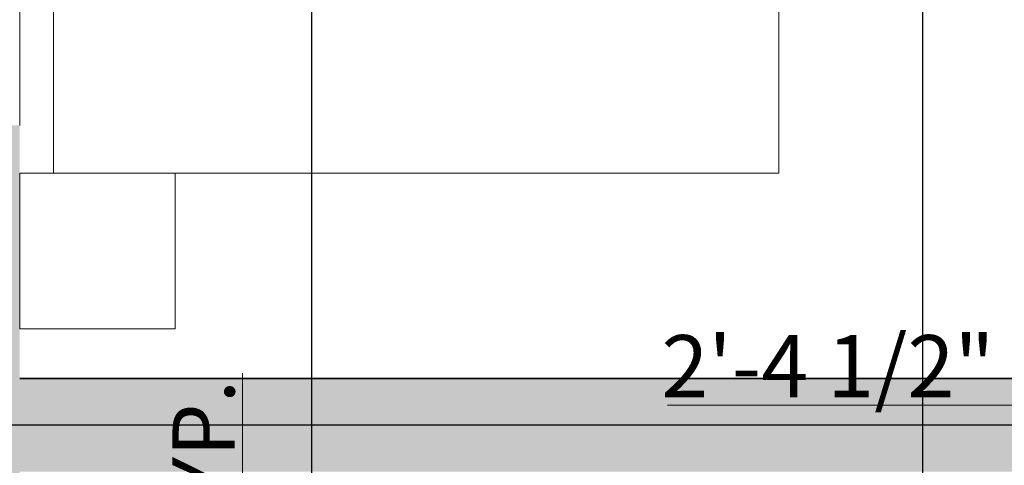
# Model space of a CAD drawing. Units: inches. Extents: x 2696 to 3240, y 1564 to 2310.
# Tile 51 of 76: x 2755 to 2850, y 2137 to 2180. Entities that reach past the tile are written whole.
import ezdxf

# ---------------------------------------------------------------- set-up
doc = ezdxf.new("R2010")
doc.units = ezdxf.units.IN
for name, color, linetype, lineweight in [('A-ANNO-DIMS', 3, 'Continuous', 18), ('A-FURN', 251, 'Continuous', 13), ('A-WALL', 7, 'Continuous', 35), ('A-WALL-PATT', 9, 'Continuous', 13), ('WINDOW', 2, 'Continuous', 18)]:
    doc.layers.add(name, color=color, linetype=linetype, lineweight=lineweight)
doc.styles.add('TIMES NEW', font='times.ttf')
doc.dimstyles.new('Siddhuu', dxfattribs={"dimtxt": 6, "dimasz": 2.5, "dimexe": 1.25, "dimexo": 0.625, "dimtad": 1, "dimdec": 1, "dimlunit": 4, "dimtxsty": 'TIMES NEW', "dimcen": 2.5, "dimclrd": 256, "dimclre": 1, "dimclrt": 7, "dimadec": 0, "dimazin": 0, "dimtfac": 1, "dimtdec": 1, "dimtmove": 0, "dimatfit": 3, "dimfxl": 1, "dimtolj": 1, "dimlwd": -1, "dimarcsym": 0})

# ---------------------------------------------------------------- blocks, each defined once
blk = doc.blocks.new('WD_WIN4')
for p, q in [((-0.5, 0.5), (0.5, 0.5)), ((-0.5, 0.12), (0.5, 0.12)), ((-0.5, -0.12), (0.5, -0.12)), ((-0.5, -0.5), (0.5, -0.5))]:
    blk.add_line(p, q)
blk = doc.blocks.new('BED-DOUBLE-WITH-NIGHTSTANDS')
for points in [[(0, 75.132), (0, 90.158), (15.027, 90.158), (15.027, 75.132)], [(3.281, 15.026), (3.281, 75.132), (73.404, 75.132), (73.404, 15.026)], [(0, 15.026), (0, 0), (15.027, 0), (15.027, 15.026)]]:
    blk.add_lwpolyline(points, close=True)
blk = doc.blocks.new('*D29')
at = {"layer": 'A-ANNO-DIMS', "color": 1, "lineweight": -2, "transparency": 16777216}
for p, q in [((2850.765, 2146.449), (2850.765, 2141.394)), ((2879.111, 2146.449), (2879.111, 2141.394))]:
    blk.add_line(p, q, dxfattribs=at)
at = {"layer": 'A-ANNO-DIMS', "transparency": 16777216}
for p, q in [((2850.765, 2142.644), (2817.236, 2142.644)), ((2876.611, 2142.644), (2853.265, 2142.644))]:
    blk.add_line(p, q, dxfattribs=at)
for points in [[(2853.265, 2143.061), (2853.265, 2142.228), (2850.765, 2142.644)], [(2876.611, 2143.061), (2876.611, 2142.228), (2879.111, 2142.644)]]:
    blk.add_solid(points, dxfattribs=at)
at = {"layer": 'Defpoints', "color": 0, "transparency": 16777216}
for p in [(2850.765, 2147.074), (2879.111, 2147.074), (2850.765, 2142.644)]:
    blk.add_point(p, dxfattribs=at)
at = {"layer": 'A-ANNO-DIMS', "color": 7, "transparency": 16777216, "insert": (2832.75, 2146.406), "char_height": 6, "attachment_point": 5, "style": 'TIMES NEW'}
blk.add_mtext('\\A1;2\'-4 1/2"', dxfattribs=at)
blk = doc.blocks.new('*D41')
at = {"layer": 'A-ANNO-DIMS', "transparency": 16777216}
for p, q in [((2776.142, 2091.201), (2776.142, 2145.728)), ((2776.142, 2087.2), (2776.142, 2088.701))]:
    blk.add_line(p, q, dxfattribs=at)
at = {"layer": 'A-ANNO-DIMS', "color": 1, "lineweight": -2, "transparency": 16777216}
for p, q in [((2776.641, 2091.201), (2774.892, 2091.201)), ((2776.641, 2084.7), (2774.892, 2084.7))]:
    blk.add_line(p, q, dxfattribs=at)
at = {"layer": 'A-ANNO-DIMS', "transparency": 16777216}
for points in [[(2775.725, 2088.701), (2776.558, 2088.701), (2776.142, 2091.201)], [(2775.725, 2087.2), (2776.558, 2087.2), (2776.142, 2084.7)]]:
    blk.add_solid(points, dxfattribs=at)
at = {"layer": 'Defpoints', "color": 0, "transparency": 16777216}
for p in [(2776.142, 2091.201), (2777.266, 2091.201), (2777.266, 2084.7)]:
    blk.add_point(p, dxfattribs=at)
at = {"layer": 'A-ANNO-DIMS', "color": 7, "transparency": 16777216, "insert": (2772.38, 2119.715), "char_height": 6, "attachment_point": 5, "rotation": 90, "style": 'TIMES NEW'}
blk.add_mtext('\\A1;0\'-6 1/2" TYP.', dxfattribs=at)
blk = doc.blocks.new('*D62')
at = {"layer": 'A-ANNO-DIMS', "color": 1, "lineweight": -2, "transparency": 16777216}
for p, q in [((2965.084, 2140.701), (2709.361, 2140.701)), ((2965.084, 2063.591), (2709.361, 2063.591))]:
    blk.add_line(p, q, dxfattribs=at)
at = {"layer": 'A-ANNO-DIMS', "transparency": 16777216}
blk.add_line((2710.611, 2066.091), (2710.611, 2138.201), dxfattribs=at)
for points in [[(2710.195, 2138.201), (2711.028, 2138.201), (2710.611, 2140.701)], [(2710.195, 2066.091), (2711.028, 2066.091), (2710.611, 2063.591)]]:
    blk.add_solid(points, dxfattribs=at)
at = {"layer": 'Defpoints', "color": 0, "transparency": 16777216}
for p in [(2710.611, 2140.701), (2965.709, 2140.701), (2965.709, 2063.591)]:
    blk.add_point(p, dxfattribs=at)
at = {"layer": 'A-ANNO-DIMS', "color": 7, "transparency": 16777216, "insert": (2706.934, 2102.146), "char_height": 6, "attachment_point": 5, "rotation": 90, "style": 'TIMES NEW'}
blk.add_mtext('\\A1;6\'-5"', dxfattribs=at)
blk = doc.blocks.new('*D64')
at = {"layer": 'A-ANNO-DIMS', "color": 1, "lineweight": -2, "transparency": 16777216}
for p, q in [((3073.084, 2206.701), (2709.361, 2206.701)), ((3068.584, 1989.201), (2709.361, 1989.201))]:
    blk.add_line(p, q, dxfattribs=at)
at = {"layer": 'A-ANNO-DIMS', "transparency": 16777216}
blk.add_line((2710.611, 1991.701), (2710.611, 2204.201), dxfattribs=at)
for points in [[(2710.195, 2204.201), (2711.028, 2204.201), (2710.611, 2206.701)], [(2710.195, 1991.701), (2711.028, 1991.701), (2710.611, 1989.201)]]:
    blk.add_solid(points, dxfattribs=at)
at = {"layer": 'Defpoints', "color": 0, "transparency": 16777216}
for p in [(2710.611, 2206.701), (3073.709, 2206.701), (3069.209, 1989.201)]:
    blk.add_point(p, dxfattribs=at)
at = {"layer": 'A-ANNO-DIMS', "color": 7, "transparency": 16777216, "insert": (2706.85, 2097.951), "char_height": 6, "attachment_point": 5, "rotation": 90, "style": 'TIMES NEW'}
blk.add_mtext('\\A1;18\'-1 1/2"', dxfattribs=at)
blk = doc.blocks.new('*D68')
at = {"layer": 'A-ANNO-DIMS', "color": 1, "lineweight": -2, "transparency": 16777216}
for p, q in [((2745.611, 2261.576), (2745.611, 1568.951)), ((2782.834, 2261.576), (2782.834, 1568.951))]:
    blk.add_line(p, q, dxfattribs=at)
at = {"layer": 'A-ANNO-DIMS', "transparency": 16777216}
blk.add_line((2748.111, 1570.201), (2780.334, 1570.201), dxfattribs=at)
for points in [[(2748.111, 1570.618), (2748.111, 1569.784), (2745.611, 1570.201)], [(2780.334, 1570.618), (2780.334, 1569.784), (2782.834, 1570.201)]]:
    blk.add_solid(points, dxfattribs=at)
at = {"layer": 'Defpoints', "color": 0, "transparency": 16777216}
for p in [(2745.611, 2262.201), (2782.834, 2262.201), (2782.834, 1570.201)]:
    blk.add_point(p, dxfattribs=at)
at = {"layer": 'A-ANNO-DIMS', "color": 7, "transparency": 16777216, "insert": (2764.223, 1573.878), "char_height": 6, "attachment_point": 5, "style": 'TIMES NEW'}
blk.add_mtext('\\A1;3\'-1"', dxfattribs=at)
blk = doc.blocks.new('*D69')
at = {"layer": 'A-ANNO-DIMS', "color": 1, "lineweight": -2, "transparency": 16777216}
for p, q in [((2841.889, 2261.576), (2841.889, 1568.951)), ((2905.91, 2261.576), (2905.91, 1568.951))]:
    blk.add_line(p, q, dxfattribs=at)
at = {"layer": 'A-ANNO-DIMS', "transparency": 16777216}
blk.add_line((2844.389, 1570.201), (2903.41, 1570.201), dxfattribs=at)
for points in [[(2844.389, 1570.618), (2844.389, 1569.784), (2841.889, 1570.201)], [(2903.41, 1570.618), (2903.41, 1569.784), (2905.91, 1570.201)]]:
    blk.add_solid(points, dxfattribs=at)
at = {"layer": 'Defpoints', "color": 0, "transparency": 16777216}
for p in [(2841.889, 2262.201), (2905.91, 2262.201), (2905.91, 1570.201)]:
    blk.add_point(p, dxfattribs=at)
at = {"layer": 'A-ANNO-DIMS', "color": 7, "transparency": 16777216, "insert": (2873.9, 1573.878), "char_height": 6, "attachment_point": 5, "style": 'TIMES NEW'}
blk.add_mtext('\\A1;5\'-4"', dxfattribs=at)

msp = doc.modelspace()

# ---------------------------------------------------------------- hatches: boundary and pattern name
at = {"layer": 'A-WALL-PATT', "transparency": 33554556}
h = msp.add_hatch(color=256, dxfattribs=at)
h.dxf.hatch_style = 1
h.paths.add_polyline_path([(2879.111, 2253.201), (2905.91, 2253.201), (2905.91, 2262.201), (2841.889, 2262.201), (2841.889, 2253.201), (2870.111, 2253.201), (2870.111, 2176.601), (2965.709, 2176.601), (2965.709, 2206.701), (2973.583, 2206.701), (2973.583, 2215.701), (2965.709, 2215.701), (2965.709, 2262.201), (2929.91, 2262.201), (2929.91, 2253.201), (2956.709, 2253.201), (2956.709, 2185.601), (2879.111, 2185.601)])
h.paths.add_polyline_path([(2782.834, 2262.201), (2745.611, 2262.201), (2745.611, 2228.729), (2754.611, 2228.729), (2754.611, 2253.201), (2782.834, 2253.201)])
h.paths.add_polyline_path([(2754.611, 2136.201), (2965.709, 2136.201), (2965.709, 2145.201), (2879.111, 2145.201), (2879.111, 2147.074), (2877.34, 2147.074), (2870.111, 2147.074), (2870.111, 2145.201), (2754.611, 2145.201), (2754.611, 2169.674), (2745.611, 2169.674), (2745.611, 2000.201), (2754.611, 2000.201), (2754.611, 2019.201), (2849.083, 2019.201), (2849.083, 2023.701), (2841.209, 2023.701), (2841.209, 2051.827), (2836.709, 2051.827), (2836.709, 2023.701), (2754.611, 2023.701), (2754.611, 2091.201), (2836.709, 2091.201), (2836.709, 2087.827), (2841.209, 2087.827), (2841.209, 2095.701), (2754.611, 2095.701)])
h.paths.add_polyline_path([(2965.709, 2136.201), (2956.709, 2136.201), (2956.709, 2023.701), (2885.083, 2023.701), (2885.083, 2019.201), (2956.709, 2019.201), (2956.709, 1950.575), (2965.709, 1950.575), (2965.709, 1980.201), (2973.583, 1980.201), (2973.583, 1989.201), (2965.709, 1989.201)])
h.paths.add_polyline_path([(2754.611, 1906.701), (2880.209, 1906.701), (2884.709, 1906.701), (2956.709, 1906.701), (2956.709, 1792.701), (2944.709, 1792.701), (2944.709, 1783.701), (2956.709, 1783.701), (2956.709, 1740.201), (2884.709, 1740.201), (2884.709, 1783.701), (2896.709, 1783.701), (2896.709, 1792.701), (2884.709, 1792.701), (2884.709, 1846.701), (2880.209, 1846.701), (2880.209, 1740.201), (2754.611, 1740.201), (2754.611, 1777.201), (2745.611, 1777.201), (2745.611, 1692.701), (2754.611, 1692.701), (2754.611, 1731.201), (2956.709, 1731.201), (2956.709, 1723.327), (2965.709, 1723.327), (2965.709, 1884.201), (2973.583, 1884.201), (2973.583, 1893.201), (2965.709, 1893.201), (2965.709, 1914.575), (2956.709, 1914.575), (2956.709, 1911.201), (2754.611, 1911.201), (2754.611, 1930.201), (2745.611, 1930.201), (2745.611, 1817.201), (2754.611, 1817.201), (2754.611, 1854.201), (2826.611, 1854.201), (2826.611, 1868.827), (2822.111, 1868.827), (2822.111, 1858.701), (2754.611, 1858.701)])
h.paths.add_polyline_path([(2965.709, 1656.201), (3008.237, 1656.201), (3008.237, 1665.201), (2965.709, 1665.201), (2965.709, 1693.327), (2956.709, 1693.327), (2956.709, 1686.201), (2934.583, 1686.201), (2934.583, 1681.701), (2956.709, 1681.701), (2956.709, 1614.201), (2896.709, 1614.201), (2896.709, 1681.701), (2904.583, 1681.701), (2904.583, 1686.201), (2892.209, 1686.201), (2892.209, 1614.201), (2858.41, 1614.201), (2858.41, 1605.201), (2965.709, 1605.201)])
h.paths.add_polyline_path([(2788.41, 1614.201), (2754.611, 1614.201), (2754.611, 1652.701), (2745.611, 1652.701), (2745.611, 1605.201), (2788.41, 1605.201)])
h.paths.add_polyline_path([(3199.611, 1633.048), (3190.611, 1633.048), (3190.611, 1614.201), (3082.611, 1614.201), (3082.611, 1665.201), (3070.237, 1665.201), (3070.237, 1656.201), (3078.111, 1656.201), (3078.111, 1605.201), (3199.611, 1605.201)])
h.paths.add_polyline_path([(3199.611, 1702.048), (3190.611, 1702.048), (3190.611, 1699.701), (3106.611, 1699.701), (3106.611, 1747.701), (3190.611, 1747.701), (3190.611, 1752.201), (3082.611, 1752.201), (3082.611, 1760.075), (3078.111, 1760.075), (3078.111, 1747.701), (3102.111, 1747.701), (3102.111, 1699.701), (3078.111, 1699.701), (3078.111, 1695.201), (3190.611, 1695.201), (3190.611, 1676.355), (3199.611, 1676.355)])
h.paths.add_polyline_path([(3199.611, 1783.201), (3190.611, 1783.201), (3190.611, 1745.355), (3199.611, 1745.355)])
h.paths.add_polyline_path([(3082.611, 1884.201), (3190.611, 1884.201), (3190.611, 1853.201), (3199.611, 1853.201), (3199.611, 1901.701), (3190.611, 1901.701), (3190.611, 1893.201), (3005.583, 1893.201), (3005.583, 1891.281), (3005.583, 1884.201), (3078.111, 1884.201), (3078.111, 1792.075), (3082.611, 1792.075)])
h.paths.add_polyline_path([(3199.611, 1994.701), (3190.611, 1994.701), (3190.611, 1989.201), (3073.709, 1989.201), (3073.709, 2034.201), (3069.209, 2034.201), (3069.209, 1989.201), (3005.583, 1989.201), (3005.583, 1980.201), (3190.611, 1980.201), (3190.611, 1971.701), (3199.611, 1971.701)])
h.paths.add_polyline_path([(3199.611, 2155.201), (3190.611, 2155.201), (3190.611, 2064.701), (3199.611, 2064.701)])
h.paths.add_polyline_path([(3190.611, 2074.701), (3106.611, 2074.701), (3106.611, 2122.701), (3190.611, 2122.701), (3190.611, 2127.201), (3082.709, 2127.201), (3082.709, 2135.075), (3073.709, 2135.075), (3073.709, 2122.701), (3102.111, 2122.701), (3102.111, 2074.701), (3069.209, 2074.701), (3069.209, 2070.201), (3190.611, 2070.201)])
h.paths.add_polyline_path([(3082.709, 2253.201), (3190.611, 2253.201), (3190.611, 2225.201), (3199.611, 2225.201), (3199.611, 2262.201), (3073.709, 2262.201), (3073.709, 2215.701), (3035.583, 2215.701), (3035.583, 2206.701), (3073.709, 2206.701), (3073.709, 2171.075), (3082.709, 2171.075)])

# ---------------------------------------------------------------- linework, layer by layer
at = {"layer": 'A-WALL'}
msp.add_line((2754.611, 2145.201), (2870.111, 2145.201), dxfattribs=at)

# ---------------------------------------------------------------- block references
at = {"layer": 'A-FURN'}
msp.add_blockref('BED-DOUBLE-WITH-NIGHTSTANDS', (2754.611, 2150.017), dxfattribs=at)
at = {"layer": 'WINDOW', "xscale": 59.05511811023622, "yscale": 8.999999999999545, "zscale": 59.05511811023622, "rotation": 269.9999999999996}
msp.add_blockref('WD_WIN4', (2750.111, 2199.201), dxfattribs=at)

# ---------------------------------------------------------------- dimensions: what is measured, and where the dimension line sits
at = {"layer": 'A-ANNO-DIMS'}
for base, p1, p2, picture, middle in [((2782.834, 1570.201), (2745.611, 2262.201), (2782.834, 2262.201), '*D68', (2764.223, 1573.878)), ((2905.91, 1570.201), (2841.889, 2262.201), (2905.91, 2262.201), '*D69', (2873.9, 1573.878))]:
    dim = msp.add_linear_dim(base=base, p1=p1, p2=p2, dimstyle='Siddhuu', override={"dimdec": 1, "dimlfac": 1, "dimrnd": 0, "dimzin": 1, "dimdsep": 46, "dimlunit": 4, "dimfrac": 2}, dxfattribs=at)
    dim.commit()
    dim.dimension.update_dxf_attribs({"geometry": picture, "text_midpoint": middle})
for base, p1, p2, angle, picture, middle in [((2710.611, 2206.701), (3069.209, 1989.201), (3073.709, 2206.701), 90, '*D64', (2706.85, 2097.951)), ((2850.765, 2142.644), (2879.111, 2147.074), (2850.765, 2147.074), 180, '*D29', (2832.75, 2146.406)), ((2710.611, 2140.701), (2965.709, 2063.591), (2965.709, 2140.701), 90, '*D62', (2706.934, 2102.146))]:
    dim = msp.add_linear_dim(base=base, p1=p1, p2=p2, angle=angle, dimstyle='Siddhuu', override={"dimdec": 1, "dimlfac": 1, "dimrnd": 0, "dimzin": 1, "dimdsep": 46, "dimlunit": 4, "dimfrac": 2}, dxfattribs=at)
    dim.commit()
    dim.dimension.update_dxf_attribs({"geometry": picture, "text_midpoint": middle})
dim = msp.add_linear_dim(base=(2776.142, 2091.201), p1=(2777.266, 2084.7), p2=(2777.266, 2091.201), angle=90, text='<> TYP.', dimstyle='Siddhuu', override={"dimdec": 1, "dimlfac": 1, "dimrnd": 0, "dimzin": 1, "dimdsep": 46, "dimlunit": 4, "dimfrac": 2}, dxfattribs=at)
dim.commit()
dim.dimension.update_dxf_attribs({"geometry": '*D41', "text_midpoint": (2772.38, 2119.715)})

doc.saveas('drawing.dxf')
